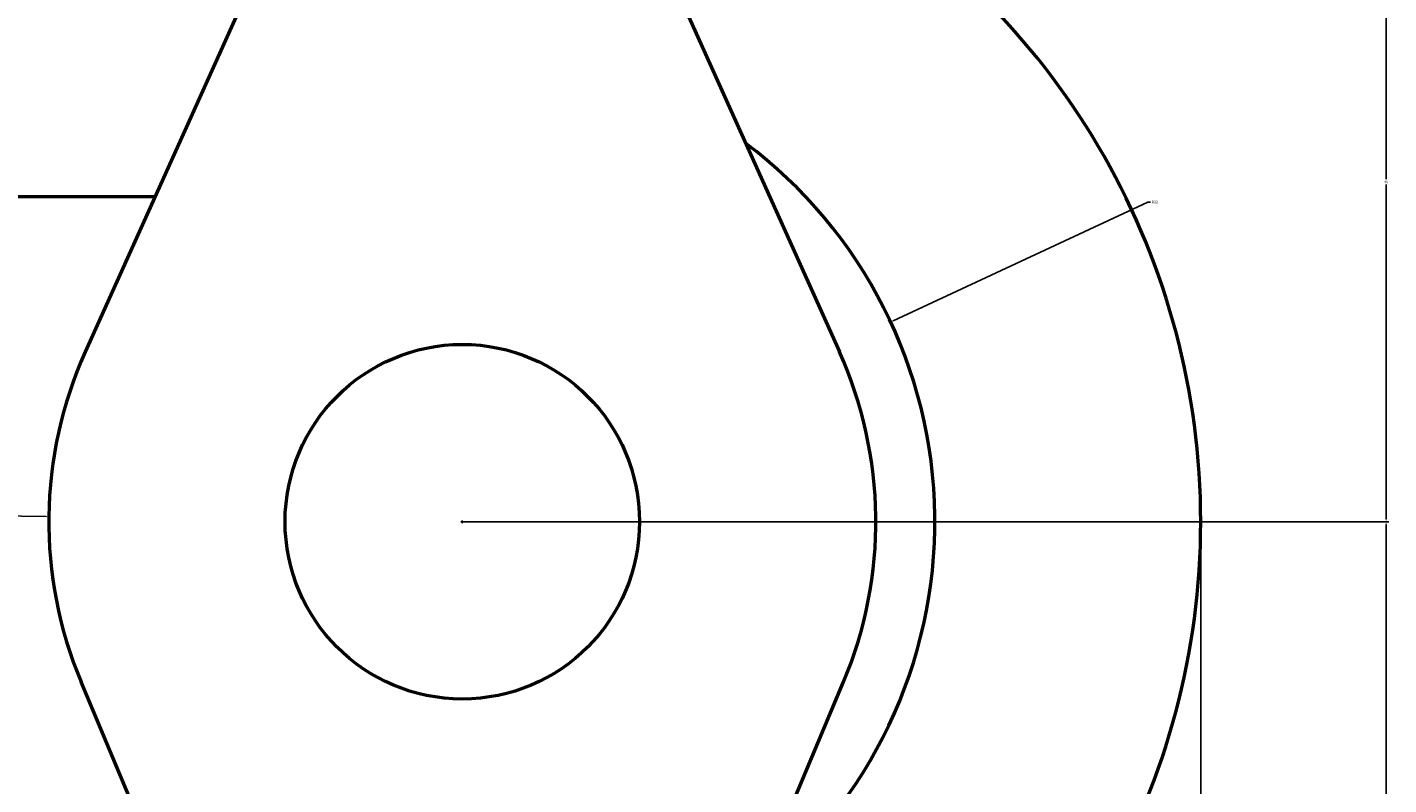
# Model space of a CAD drawing. Units: inches. Extents: x -307 to -76, y 16 to 196.
# Tile 6 of 7: x -168 to -76, y 83 to 134. Entities that reach past the tile are written whole.
import ezdxf

# ---------------------------------------------------------------- set-up
doc = ezdxf.new("R2010")
doc.units = ezdxf.units.IN
doc.header["$MEASUREMENT"] = 0
for name, color, linetype, lineweight in [('M-DIMS', 2, 'Continuous', 18), ('M-OUTL', 7, 'Continuous', 50), ('M-OUTL-LINK', 7, 'Continuous', 50)]:
    doc.layers.add(name, color=color, linetype=linetype, lineweight=lineweight)
doc.styles.get("Standard").update_dxf_attribs({"font": 'arial.ttf'})
doc.dimstyles.get("Standard").update_dxf_attribs({"dimtxt": 0.18, "dimasz": 0.18, "dimexe": 0.18, "dimexo": 0.0625, "dimgap": 0.09, "dimtad": 0, "dimtih": 1, "dimtoh": 1, "dimdec": 4, "dimzin": 0, "dimdsep": 46, "dimtxsty": 'Standard', "dimcen": 0.09, "dimadec": 0, "dimazin": 0, "dimtfac": 1, "dimtdec": 4, "dimtofl": 0, "dimtmove": 0, "dimatfit": 3, "dimfxl": 1, "dimtolj": 1, "dimtzin": 0, "dimarcsym": 0})

# ---------------------------------------------------------------- blocks, each defined once
blk = doc.blocks.new('*D2')
at = {"layer": 'Defpoints', "color": 0, "transparency": 16777216}
for p in [(-294.39, 101), (-88.39, 101), (-88.39, 16.45)]:
    blk.add_point(p, dxfattribs=at)
at = {"layer": 'M-DIMS', "color": 0, "lineweight": -2, "transparency": 16777216}
for p, q in [((-294.39, 100.938), (-294.39, 16.27)), ((-88.39, 100.938), (-88.39, 16.27)), ((-294.21, 16.45), (-191.68, 16.45)), ((-88.57, 16.45), (-191.099, 16.45))]:
    blk.add_line(p, q, dxfattribs=at)
at = {"layer": 'M-DIMS', "color": 0, "transparency": 16777216}
for points in [[(-294.21, 16.48), (-294.21, 16.42), (-294.39, 16.45)], [(-88.57, 16.48), (-88.57, 16.42), (-88.39, 16.45)]]:
    blk.add_solid(points, dxfattribs=at)
at = {"layer": 'M-DIMS', "color": 0, "transparency": 16777216, "insert": (-191.39, 16.45), "char_height": 0.18, "attachment_point": 5}
blk.add_mtext('\\A1;206', dxfattribs=at)
blk = doc.blocks.new('*D5')
at = {"layer": 'Defpoints', "color": 0, "transparency": 16777216}
for p in [(-138.39, 185.55), (-138.39, 157), (-203.39, 101)]:
    blk.add_point(p, dxfattribs=at)
at = {"layer": 'M-DIMS', "color": 0, "lineweight": -2, "transparency": 16777216}
for p, q in [((-203.39, 101.062), (-203.39, 185.73)), ((-203.21, 185.55), (-171.11, 185.55)), ((-138.57, 185.55), (-170.67, 185.55)), ((-138.39, 157.062), (-138.39, 185.73))]:
    blk.add_line(p, q, dxfattribs=at)
at = {"layer": 'M-DIMS', "color": 0, "transparency": 16777216}
for points in [[(-203.21, 185.58), (-203.21, 185.52), (-203.39, 185.55)], [(-138.57, 185.58), (-138.57, 185.52), (-138.39, 185.55)]]:
    blk.add_solid(points, dxfattribs=at)
at = {"layer": 'M-DIMS', "color": 0, "transparency": 16777216, "insert": (-170.89, 185.55), "char_height": 0.18, "attachment_point": 5}
blk.add_mtext('\\A1;65', dxfattribs=at)
blk = doc.blocks.new('*D8')
at = {"layer": 'Defpoints', "color": 0, "transparency": 16777216}
for p in [(-138.39, 101), (-75.84, 101), (-138.39, 55)]:
    blk.add_point(p, dxfattribs=at)
at = {"layer": 'M-DIMS', "color": 0, "lineweight": -2, "transparency": 16777216}
for p, q in [((-138.327, 101), (-75.66, 101)), ((-75.84, 100.82), (-75.84, 78.182)), ((-75.84, 55.18), (-75.84, 77.818)), ((-138.327, 55), (-75.66, 55))]:
    blk.add_line(p, q, dxfattribs=at)
at = {"layer": 'M-DIMS', "color": 0, "transparency": 16777216}
for points in [[(-75.87, 100.82), (-75.81, 100.82), (-75.84, 101)], [(-75.87, 55.18), (-75.81, 55.18), (-75.84, 55)]]:
    blk.add_solid(points, dxfattribs=at)
at = {"layer": 'M-DIMS', "color": 0, "transparency": 16777216, "insert": (-75.84, 78), "char_height": 0.18, "attachment_point": 5}
blk.add_mtext('\\A1;46', dxfattribs=at)
blk = doc.blocks.new('*D9')
at = {"layer": 'Defpoints', "color": 0, "transparency": 16777216}
for p in [(-138.39, 147), (-75.84, 147), (-138.39, 101)]:
    blk.add_point(p, dxfattribs=at)
at = {"layer": 'M-DIMS', "color": 0, "lineweight": -2, "transparency": 16777216}
for p, q in [((-138.327, 147), (-75.66, 147)), ((-75.84, 146.82), (-75.84, 124.182)), ((-75.84, 101.18), (-75.84, 123.818)), ((-138.327, 101), (-75.66, 101))]:
    blk.add_line(p, q, dxfattribs=at)
at = {"layer": 'M-DIMS', "color": 0, "transparency": 16777216}
for points in [[(-75.87, 146.82), (-75.81, 146.82), (-75.84, 147)], [(-75.87, 101.18), (-75.81, 101.18), (-75.84, 101)]]:
    blk.add_solid(points, dxfattribs=at)
at = {"layer": 'M-DIMS', "color": 0, "transparency": 16777216, "insert": (-75.84, 124), "char_height": 0.18, "attachment_point": 5}
blk.add_mtext('\\A1;46', dxfattribs=at)
blk = doc.blocks.new('*D13')
at = {"layer": 'Defpoints', "color": 0, "transparency": 16777216}
for p in [(-109.386, 114.521), (-138.39, 101)]:
    blk.add_point(p, dxfattribs=at)
at = {"layer": 'M-DIMS', "color": 0, "lineweight": -2, "transparency": 16777216}
for p, q in [((-91.984, 122.633), (-109.223, 114.597)), ((-91.804, 122.633), (-91.984, 122.633)), ((-138.48, 101), (-138.3, 101)), ((-138.39, 100.91), (-138.39, 101.09))]:
    blk.add_line(p, q, dxfattribs=at)
at = {"layer": 'M-DIMS', "color": 0, "transparency": 16777216}
blk.add_solid([(-109.236, 114.624), (-109.211, 114.57), (-109.386, 114.521)], dxfattribs=at)
at = {"layer": 'M-DIMS', "color": 0, "transparency": 16777216, "insert": (-91.5, 122.633), "char_height": 0.18, "attachment_point": 5}
blk.add_mtext('\\A1;R32', dxfattribs=at)
blk = doc.blocks.new('*D14')
at = {"layer": 'Defpoints', "color": 0, "transparency": 16777216}
for p in [(-166.387, 101.354), (-138.39, 101)]:
    blk.add_point(p, dxfattribs=at)
at = {"layer": 'M-DIMS', "color": 0, "lineweight": -2, "transparency": 16777216}
for p, q in [((-183.186, 101.566), (-166.567, 101.356)), ((-138.48, 101), (-138.3, 101)), ((-138.39, 100.91), (-138.39, 101.09))]:
    blk.add_line(p, q, dxfattribs=at)
at = {"layer": 'M-DIMS', "color": 0, "transparency": 16777216}
blk.add_solid([(-166.567, 101.386), (-166.568, 101.326), (-166.387, 101.354)], dxfattribs=at)
at = {"layer": 'M-DIMS', "color": 0, "transparency": 16777216, "insert": (-183.686, 101.566), "char_height": 0.18, "attachment_point": 5}
blk.add_mtext('\\A1;2X R28', dxfattribs=at)

msp = doc.modelspace()

# ---------------------------------------------------------------- linework, layer by layer
at = {"layer": 'M-OUTL'}
msp.add_line((-244.39, 123), (-159.193, 123), dxfattribs=at)
for radius, start, end in [(50, 300.71777, 59.28223), (32, 308.26001, 53.18884)]:
    msp.add_arc((-138.39, 101), radius, start, end, dxfattribs=at)
at = {"layer": 'M-OUTL-LINK'}
for p, q in [((-148.39, 147), (-163.922, 112.493)), ((-128.39, 147), (-112.857, 112.493)), ((-148.162, 51.964), (-164.205, 90.156)), ((-128.617, 51.964), (-112.575, 90.156))]:
    msp.add_line(p, q, dxfattribs=at)
msp.add_circle((-138.39, 101), 12, dxfattribs=at)
for start, end in [(155.76618, 202.78497), (337.21503, 24.23382)]:
    msp.add_arc((-138.39, 101), 28, start, end, dxfattribs=at)

# ---------------------------------------------------------------- dimensions: what is measured, and where the dimension line sits
at = {"layer": 'M-DIMS'}
for base, p1, p2, picture, middle in [((-138.39, 185.55), (-203.39, 101), (-138.39, 157), '*D5', (-170.89, 185.55)), ((-88.39, 16.45), (-294.39, 101), (-88.39, 101), '*D2', (-191.39, 16.45))]:
    dim = msp.add_linear_dim(base=base, p1=p1, p2=p2, dimstyle='Standard', override={"dimdec": 0, "dimlfac": 1, "dimrnd": 0, "dimzin": 0, "dimdsep": 46, "dimlunit": 2}, dxfattribs=at)
    dim.commit()
    dim.dimension.update_dxf_attribs({"geometry": picture, "text_midpoint": middle})
for base, p1, p2, picture, middle in [((-75.84, 147), (-138.39, 101), (-138.39, 147), '*D9', (-75.84, 124)), ((-75.84, 101), (-138.39, 55), (-138.39, 101), '*D8', (-75.84, 78))]:
    dim = msp.add_linear_dim(base=base, p1=p1, p2=p2, angle=90, dimstyle='Standard', override={"dimdec": 0, "dimlfac": 1, "dimrnd": 0, "dimzin": 0, "dimdsep": 46, "dimlunit": 2}, dxfattribs=at)
    dim.commit()
    dim.dimension.update_dxf_attribs({"geometry": picture, "text_midpoint": middle})
dim = msp.add_radius_dim(center=(-138.39, 101), mpoint=(-109.386, 114.521), dimstyle='Standard', override={"dimdec": 0, "dimlfac": 1, "dimrnd": 0, "dimzin": 0, "dimdsep": 46, "dimlunit": 2}, dxfattribs=at)
dim.commit()
dim.dimension.update_dxf_attribs({"geometry": '*D13', "text_midpoint": (-91.5, 122.633), "dimtype": 164})
dim = msp.add_radius_dim(center=(-138.39, 101), mpoint=(-166.387, 101.354), text='2X <>', dimstyle='Standard', override={"dimdec": 0, "dimlfac": 1, "dimrnd": 0, "dimzin": 0, "dimdsep": 46, "dimlunit": 2}, dxfattribs=at)
dim.commit()
dim.dimension.update_dxf_attribs({"geometry": '*D14', "text_midpoint": (-183.186, 101.566), "dimtype": 164})

doc.saveas('drawing.dxf')
